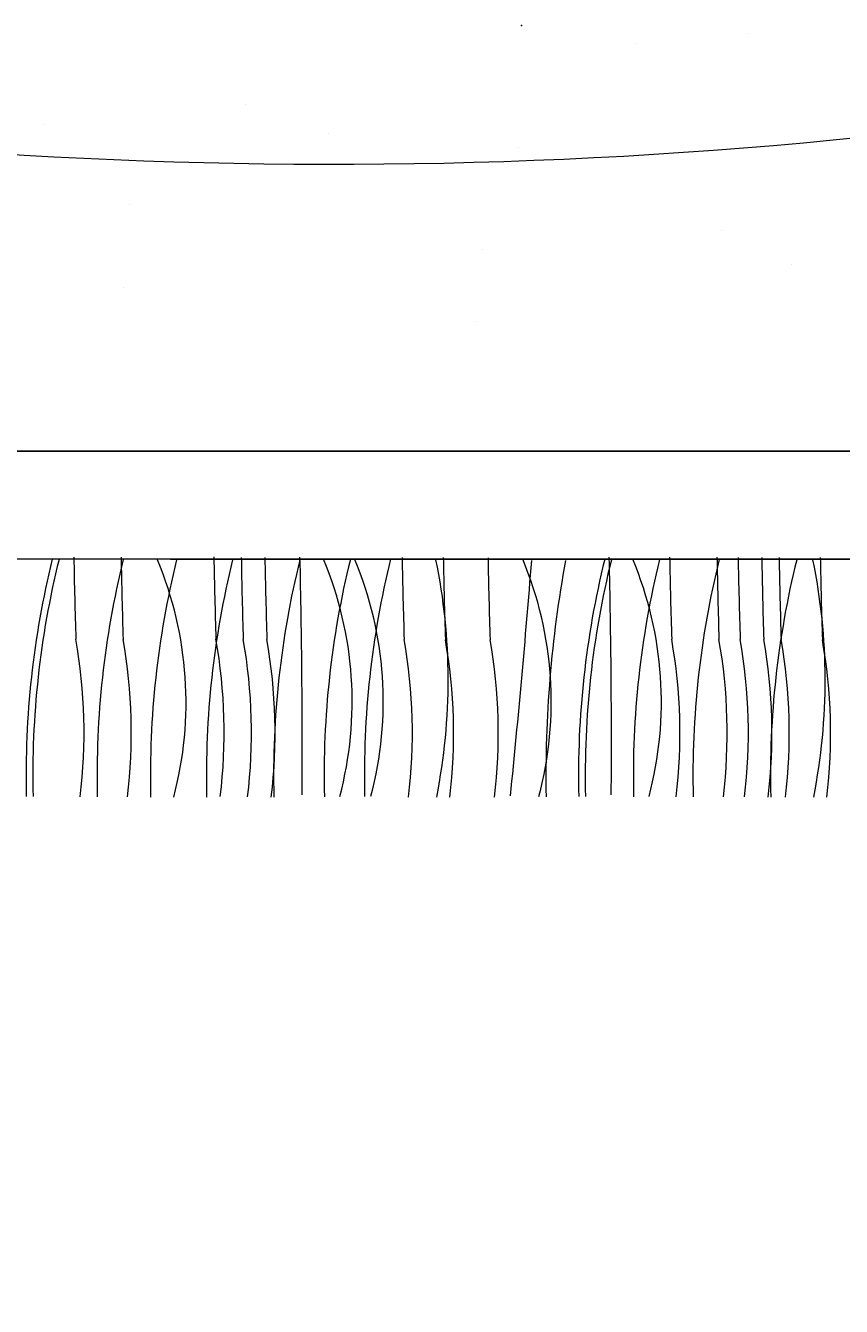
# Model space of a CAD drawing. Units: inches. Extents: x 182 to 1022, y -617 to 111.
# Tile 4 of 33: x 294 to 313, y -309 to -278. Entities that reach past the tile are written whole.
import ezdxf

# ---------------------------------------------------------------- set-up
doc = ezdxf.new("R2010")
doc.units = ezdxf.units.IN
doc.header["$MEASUREMENT"] = 0
doc.layers.add('A-ANNO-DIMS', color=2, linetype='Continuous', lineweight=18)
doc.layers.add('furniture', color=50, linetype='Continuous', lineweight=15, transparency=0.8)
doc.styles.get("Standard").update_dxf_attribs({"font": 'arial.ttf'})
doc.dimstyles.get("Standard").update_dxf_attribs({"dimtxt": 0.18, "dimasz": 0.18, "dimexe": 0.18, "dimexo": 0.0625, "dimgap": 0.09, "dimtad": 0, "dimtih": 1, "dimtoh": 1, "dimdec": 1, "dimzin": 0, "dimdsep": 46, "dimlunit": 4, "dimtxsty": 'Standard', "dimcen": 0.09, "dimadec": 0, "dimazin": 0, "dimtfac": 1, "dimtdec": 1, "dimtofl": 0, "dimtmove": 0, "dimatfit": 3, "dimfxl": 1, "dimtolj": 1, "dimtzin": 0, "dimarcsym": 0})

# ---------------------------------------------------------------- blocks, each defined once
blk = doc.blocks.new('LOUNGE-SEATING-GROUP')
for p, q in [((53.25, 18.266), (53.25, 18.266)), ((50.58, 18.039), (50.58, 18.039)), ((41.23, 16.584), (41.23, 16.584)), ((36.416, 16.105), (36.416, 16.105)), ((36.416, 16.105), (36.416, 16.105)), ((43.231, 15.882), (43.231, 15.882)), ((47.776, 15.553), (47.776, 15.553)), ((38.459, 14.179), (38.459, 14.179)), ((52.629, 13.55), (52.629, 13.55)), ((46.905, 13.103), (46.905, 13.103)), ((54.307, 12.737), (54.307, 12.737)), ((38.314, 12.188), (38.314, 12.188)), ((46.774, 11.394), (46.774, 11.394)), ((134.145, 5.694), (21.664, 5.694)), ((39.442, 5.694), (134.145, 5.694))]:
    blk.add_line(p, q)
for centre, radius, start, end in [((43.304, 138.877), 123.732, 259.92753, 281.22459), ((57.542, 0.532), 21.554, 166.1427, 181.3669), ((57.703, 0.531), 21.554, 166.1427, 181.3669), ((179.822, 8.292), 142.714, 181.02248, 181.81091), ((59.241, 0.526), 21.554, 166.1427, 181.3669), ((180.953, 8.289), 142.714, 181.02248, 181.81091), ((60.516, 0.516), 21.554, 166.1427, 181.3669), ((30.979, 2.27), 8.837, 345.1387, 22.6902), ((61.856, 0.518), 21.554, 166.1427, 181.3669), ((183.173, 8.298), 142.714, 181.02248, 181.81091), ((183.827, 8.287), 142.714, 181.02248, 181.81091), ((184.392, 8.286), 142.714, 181.02248, 181.81091), ((63.464, 0.521), 21.554, 166.1427, 181.3669), ((-141.927, 1.329), 184.521, 359.60659, 1.37204), ((34.952, 2.285), 8.837, 345.1387, 22.6902), ((64.672, 0.53), 21.554, 166.1427, 181.3669), ((35.695, 2.293), 8.837, 345.1387, 22.6902), ((65.635, 0.538), 21.554, 166.1427, 181.3669), ((187.675, 8.285), 142.714, 181.02248, 181.81091), ((31.753, 2.803), 14.333, 348.7545, 11.5888), ((188.661, 8.282), 142.714, 181.02248, 181.81091), ((189.73, 8.279), 142.714, 181.02248, 181.81091), ((-202.731, 25.472), 251.596, 354.19829, 355.48538), ((39.716, 2.289), 8.837, 345.1387, 22.6902), ((77.043, 0.5), 28.62, 169.5961, 180.9805), ((70.757, 0.532), 21.554, 166.1427, 181.3669), ((70.918, 0.531), 21.554, 166.1427, 181.3669), ((-134.53, 1.329), 184.521, 359.60659, 1.37204), ((42.349, 2.285), 8.837, 345.1387, 22.6902), ((72.069, 0.53), 21.554, 166.1427, 181.3669), ((194.075, 8.292), 142.714, 181.02248, 181.81091), ((73.495, 0.526), 21.554, 166.1427, 181.3669), ((195.206, 8.289), 142.714, 181.02248, 181.81091), ((195.713, 8.287), 142.714, 181.02248, 181.81091), ((196.277, 8.286), 142.714, 181.02248, 181.81091), ((75.349, 0.521), 21.554, 166.1427, 181.3669), ((196.692, 8.285), 142.714, 181.02248, 181.81091), ((40.771, 2.803), 14.333, 348.7545, 11.5888), ((197.679, 8.282), 142.714, 181.02248, 181.81091), ((24.582, 1.546), 12.794, 353.1171, 10.0651), ((25.712, 1.543), 12.794, 353.1171, 10.0651), ((27.933, 1.552), 12.794, 353.1171, 10.0651), ((28.587, 1.542), 12.794, 353.1171, 10.0651), ((29.152, 1.54), 12.794, 353.1171, 10.0651), ((32.435, 1.539), 12.794, 353.1171, 10.0651), ((33.421, 1.536), 12.794, 353.1171, 10.0651), ((34.49, 1.534), 12.794, 353.1171, 10.0651), ((38.835, 1.546), 12.794, 353.1171, 10.0651), ((39.966, 1.543), 12.794, 353.1171, 10.0651), ((40.473, 1.542), 12.794, 353.1171, 10.0651), ((41.037, 1.54), 12.794, 353.1171, 10.0651), ((41.452, 1.539), 12.794, 353.1171, 10.0651), ((42.439, 1.536), 12.794, 353.1171, 10.0651)]:
    blk.add_arc(centre, radius, start, end)
blk.add_point((47.843, 18.461))
blk = doc.blocks.new('*D26')
at = {"layer": 'A-ANNO-DIMS', "color": 0, "lineweight": -2, "transparency": 16777216}
for p, q in [((257.848, -296.884), (257.848, -319.733)), ((409.388, -296.884), (409.388, -319.733)), ((258.028, -319.553), (331.642, -319.553)), ((409.208, -319.553), (335.594, -319.553))]:
    blk.add_line(p, q, dxfattribs=at)
at = {"layer": 'A-ANNO-DIMS', "color": 0, "transparency": 16777216}
for points in [[(258.028, -319.523), (258.028, -319.583), (257.848, -319.553)], [(409.208, -319.523), (409.208, -319.583), (409.388, -319.553)]]:
    blk.add_solid(points, dxfattribs=at)
at = {"layer": 'Defpoints', "color": 0, "transparency": 16777216}
for p in [(257.848, -296.822), (409.388, -296.822), (409.388, -319.553)]:
    blk.add_point(p, dxfattribs=at)
at = {"layer": 'A-ANNO-DIMS', "color": 0, "transparency": 16777216, "insert": (333.618, -319.553), "char_height": 0.18, "attachment_point": 5}
blk.add_mtext('\\A1;LOUNGE GROUP 12\'-7 1/2" TYP.', dxfattribs=at)
blk = doc.blocks.new('*D39')
at = {"layer": 'A-ANNO-DIMS', "color": 0, "lineweight": -2, "transparency": 16777216}
for p, q in [((238.398, -288.54), (1015.285, -288.54)), ((1015.105, -288.72), (1015.105, -346.775)), ((1015.105, -405.193), (1015.105, -347.138)), ((238.427, -405.373), (1015.285, -405.373))]:
    blk.add_line(p, q, dxfattribs=at)
at = {"layer": 'A-ANNO-DIMS', "color": 0, "transparency": 16777216}
for points in [[(1015.075, -288.72), (1015.135, -288.72), (1015.105, -288.54)], [(1015.075, -405.193), (1015.135, -405.193), (1015.105, -405.373)]]:
    blk.add_solid(points, dxfattribs=at)
at = {"layer": 'Defpoints', "color": 0, "transparency": 16777216}
for p in [(238.335, -288.54), (1015.105, -288.54), (238.364, -405.373)]:
    blk.add_point(p, dxfattribs=at)
at = {"layer": 'A-ANNO-DIMS', "color": 0, "transparency": 16777216, "insert": (1015.105, -346.956), "char_height": 0.18, "attachment_point": 5}
blk.add_mtext('\\A1;9\'-9"', dxfattribs=at)

msp = doc.modelspace()

# ---------------------------------------------------------------- block references
at = {"layer": 'furniture'}
msp.add_blockref('LOUNGE-SEATING-GROUP', (257.848, -296.822), dxfattribs=at)

# ---------------------------------------------------------------- dimensions: what is measured, and where the dimension line sits
at = {"layer": 'A-ANNO-DIMS'}
dim = msp.add_linear_dim(base=(1015.105, -288.54), p1=(238.364, -405.373), p2=(238.335, -288.54), angle=90, dimstyle='Standard', override={"dimdec": 1, "dimlfac": 1, "dimrnd": 0, "dimzin": 1, "dimdsep": 46, "dimlunit": 4, "dimfrac": 2}, dxfattribs=at)
dim.commit()
dim.dimension.update_dxf_attribs({"geometry": '*D39', "text_midpoint": (1015.105, -346.956)})
dim = msp.add_linear_dim(base=(409.388, -319.553), p1=(257.848, -296.822), p2=(409.388, -296.822), text='LOUNGE GROUP <> TYP.', dimstyle='Standard', override={"dimdec": 1, "dimlfac": 1, "dimrnd": 0, "dimzin": 1, "dimdsep": 46, "dimlunit": 4, "dimfrac": 2}, dxfattribs=at)
dim.commit()
dim.dimension.update_dxf_attribs({"geometry": '*D26', "text_midpoint": (333.618, -319.553)})

doc.saveas('drawing.dxf')
